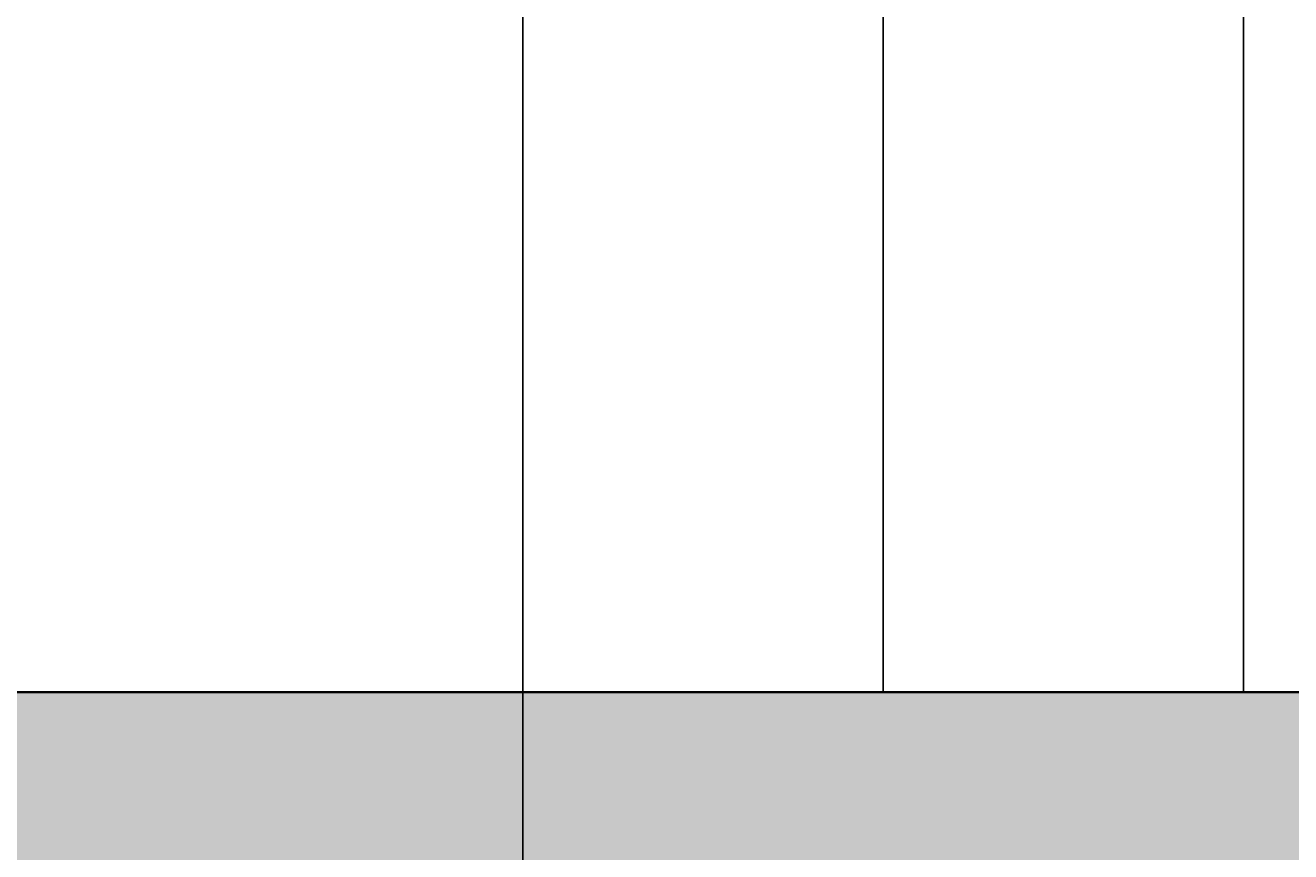
# Model space of a CAD drawing. Units: inches. Extents: x 1998 to 2588, y 1139 to 1977.
# Tile 87 of 134: x 2397 to 2425, y 1477 to 1496. Entities that reach past the tile are written whole.
import ezdxf

# ---------------------------------------------------------------- set-up
doc = ezdxf.new("R2010")
doc.units = ezdxf.units.IN
for name, color, linetype, lineweight in [('A-ANNO-DIMS', 2, 'Continuous', 18), ('A-FLOR-STRS', 7, 'Continuous', 25), ('A-WALL-PATT', 252, 'Continuous', 13), ('WALL', 200, 'Continuous', 35)]:
    doc.layers.add(name, color=color, linetype=linetype, lineweight=lineweight)
doc.styles.get("Standard").update_dxf_attribs({"font": 'arial.ttf'})
doc.dimstyles.get("Standard").update_dxf_attribs({"dimtxt": 0.18, "dimasz": 0.18, "dimexe": 0.18, "dimexo": 0.0625, "dimgap": 0.09, "dimtad": 0, "dimtih": 1, "dimtoh": 1, "dimdec": 4, "dimzin": 0, "dimdsep": 46, "dimtxsty": 'Standard', "dimcen": 0.09, "dimadec": 0, "dimazin": 0, "dimtfac": 1, "dimtdec": 4, "dimtofl": 0, "dimtmove": 0, "dimatfit": 3, "dimfxl": 1, "dimtolj": 1, "dimtzin": 0, "dimarcsym": 0})

# ---------------------------------------------------------------- blocks, each defined once
blk = doc.blocks.new('*D24')
at = {"layer": 'A-ANNO-DIMS', "color": 0, "lineweight": -2, "transparency": 16777216}
for p, q in [((2398.535, 1911.232), (2588.309, 1911.232)), ((2588.129, 1911.052), (2588.129, 1570.164)), ((2588.129, 1228.912), (2588.129, 1569.8)), ((2527.535, 1228.732), (2588.309, 1228.732))]:
    blk.add_line(p, q, dxfattribs=at)
at = {"layer": 'A-ANNO-DIMS', "color": 0, "transparency": 16777216}
for points in [[(2588.099, 1911.052), (2588.159, 1911.052), (2588.129, 1911.232)], [(2588.099, 1228.912), (2588.159, 1228.912), (2588.129, 1228.732)]]:
    blk.add_solid(points, dxfattribs=at)
at = {"layer": 'Defpoints', "color": 0, "transparency": 16777216}
for p in [(2398.473, 1911.232), (2588.129, 1911.232), (2527.473, 1228.732)]:
    blk.add_point(p, dxfattribs=at)
at = {"layer": 'A-ANNO-DIMS', "color": 0, "transparency": 16777216, "insert": (2588.129, 1569.982), "char_height": 0.18, "attachment_point": 5}
blk.add_mtext('\\A1;682.5', dxfattribs=at)
blk = doc.blocks.new('*D33')
at = {"layer": 'A-ANNO-DIMS', "color": 0, "lineweight": -2, "transparency": 16777216}
for p, q in [((2407.973, 1480.67), (2407.973, 1138.602)), ((2498.179, 1480.67), (2498.179, 1138.602)), ((2408.153, 1138.782), (2452.753, 1138.782)), ((2497.999, 1138.782), (2453.399, 1138.782))]:
    blk.add_line(p, q, dxfattribs=at)
at = {"layer": 'A-ANNO-DIMS', "color": 0, "transparency": 16777216}
for points in [[(2408.153, 1138.812), (2408.153, 1138.752), (2407.973, 1138.782)], [(2497.999, 1138.812), (2497.999, 1138.752), (2498.179, 1138.782)]]:
    blk.add_solid(points, dxfattribs=at)
at = {"layer": 'Defpoints', "color": 0, "transparency": 16777216}
for p in [(2407.973, 1480.732), (2498.179, 1480.732), (2498.179, 1138.782)]:
    blk.add_point(p, dxfattribs=at)
at = {"layer": 'A-ANNO-DIMS', "color": 0, "transparency": 16777216, "insert": (2453.076, 1138.782), "char_height": 0.18, "attachment_point": 5}
blk.add_mtext('\\A1;90.2', dxfattribs=at)
blk = doc.blocks.new('*D43')
at = {"layer": 'A-ANNO-DIMS', "color": 0, "lineweight": -2, "transparency": 16777216}
for p, q in [((2407.973, 1594.67), (2407.973, 1138.602)), ((2345.973, 1588.67), (2345.973, 1138.602)), ((2346.153, 1138.782), (2376.754, 1138.782)), ((2407.793, 1138.782), (2377.191, 1138.782))]:
    blk.add_line(p, q, dxfattribs=at)
at = {"layer": 'A-ANNO-DIMS', "color": 0, "transparency": 16777216}
for points in [[(2346.153, 1138.812), (2346.153, 1138.752), (2345.973, 1138.782)], [(2407.793, 1138.812), (2407.793, 1138.752), (2407.973, 1138.782)]]:
    blk.add_solid(points, dxfattribs=at)
at = {"layer": 'Defpoints', "color": 0, "transparency": 16777216}
for p in [(2407.973, 1594.732), (2345.973, 1588.732), (2407.973, 1138.782)]:
    blk.add_point(p, dxfattribs=at)
at = {"layer": 'A-ANNO-DIMS', "color": 0, "transparency": 16777216, "insert": (2376.973, 1138.782), "char_height": 0.18, "attachment_point": 5}
blk.add_mtext('\\A1;62', dxfattribs=at)

msp = doc.modelspace()

# ---------------------------------------------------------------- hatches: boundary and pattern name
at = {"layer": 'A-WALL-PATT'}
h = msp.add_hatch(color=256, dxfattribs=at)
h.dxf.hatch_style = 1
h.paths.add_polyline_path([(2527.4729, 1362.2324), (2510.9729, 1362.2324), (2510.9729, 1357.7324), (2518.4729, 1357.7324), (2518.4729, 1237.7324), (2503.1458, 1237.7324), (2503.1458, 1228.7324), (2527.4729, 1228.7324)])
h.paths.add_polyline_path([(2490.5682, 1362.2324), (2398.4729, 1362.2324), (2398.4729, 1357.7324), (2490.5682, 1357.7324)])
h.paths.add_polyline_path([(2224.9729, 1264.7324), (2222.9729, 1264.7324), (2222.9729, 1232.4125), (2341.4729, 1232.4125), (2341.4729, 1234.4125), (2224.9729, 1234.4125)])
h.paths.add_polyline_path([(2334.5332, 1273.7324), (2264.7638, 1273.7324), (2264.7638, 1269.5611, -0.043659), (2264.3413, 1264.7324), (2334.5332, 1264.7324)])
h.paths.add_polyline_path([(2236.9551, 1273.7324), (2234.4125, 1273.7324), (2234.4125, 1264.7324), (2236.9551, 1264.7324), (2236.9551, 1269.5611)])
h.paths.add_polyline_path([(2222.9729, 1293.2324), (2096.9729, 1293.2324), (2096.9729, 1345.0966), (2087.9729, 1345.0966), (2087.9729, 1284.2324), (2222.9729, 1284.2324), (2222.9729, 1285.137)])
h.paths.add_polyline_path([(2096.9729, 1458.7927), (2087.9729, 1458.7927), (2087.9729, 1417.7324), (2087.9729, 1413.2324), (2096.9729, 1413.2324), (2096.9729, 1417.7324)])
h.paths.add_polyline_path([(2096.9729, 1413.2324), (2087.9729, 1413.2324), (2087.9729, 1365.5012), (2096.9729, 1365.5012), (2096.9729, 1369.3358)])
h.paths.add_polyline_path([(2186.2943, 1417.7324), (2138.6074, 1417.7324), (2096.9729, 1417.7324), (2096.9729, 1413.2324), (2138.6074, 1413.2324), (2186.2943, 1413.2324)])
h.paths.add_polyline_path([(2181.4729, 1465.7324), (2176.9729, 1465.7324), (2176.9729, 1451.6434), (2181.4729, 1451.6434)])
h.paths.add_polyline_path([(2181.4729, 1422.1664), (2176.9729, 1422.1664), (2176.9729, 1417.7324), (2181.4729, 1417.7324)])
h.paths.add_polyline_path([(2063.9729, 1465.7324), (2087.9729, 1465.7324), (2087.9729, 1470.2324), (2059.4729, 1470.2324), (2059.4729, 1413.2324), (2087.9729, 1413.2324), (2087.9729, 1417.7324), (2063.9729, 1417.7324)])
h.paths.add_polyline_path([(2181.4729, 1755.2324), (2176.9729, 1755.2324), (2176.9729, 1748.6798), (2177.0513, 1748.6798), (2181.4729, 1748.6798)])
h.paths.add_polyline_path([(2227.4729, 1707.2324), (2220.4647, 1707.2324), (2220.4647, 1702.7324), (2222.9729, 1702.7324), (2222.9729, 1604.637), (2227.4729, 1604.637)])
h.paths.add_polyline_path([(2114.9729, 1702.7324), (2105.9729, 1702.7324), (2105.9729, 1628.4781, -0.0318759), (2110.1012, 1628.7416), (2114.9729, 1628.7416)])
h.paths.add_polyline_path([(2345.9729, 1739.3278), (2341.4729, 1739.3278), (2341.4729, 1647.5211), (2345.9729, 1647.5211)])
h.paths.add_polyline_path([(2350.6273, 1641.2324), (2345.9729, 1641.2324), (2345.9729, 1636.7324), (2350.6273, 1636.7324), (2350.6273, 1639.8729)])
h.paths.add_polyline_path([(2501.9729, 1641.2324), (2407.9729, 1641.2324), (2392.5005, 1641.2324), (2392.5005, 1639.8729), (2392.5005, 1636.7324), (2501.9729, 1636.7324)])
h.paths.add_polyline_path([(2510.9729, 1755.2324), (2501.9729, 1755.2324), (2501.9729, 1641.2324), (2510.9729, 1641.2324)])
h.paths.add_polyline_path([(2549.1786, 1641.2324), (2522.3775, 1641.2324), (2522.3775, 1636.7324), (2540.1786, 1636.7324), (2540.1786, 1480.7324), (2522.3775, 1480.7324), (2522.3775, 1476.2324), (2549.1786, 1476.2324)])
h.paths.add_polyline_path([(2498.1786, 1594.7324), (2407.9729, 1594.7324), (2407.9729, 1585.7324), (2416.9729, 1585.7324), (2489.1786, 1585.7324), (2489.1786, 1531.7324), (2416.9729, 1531.7324), (2407.9729, 1531.7324), (2407.9729, 1522.7324), (2498.1786, 1522.7324)])
h.paths.add_polyline_path([(2351.6437, 1480.7324), (2345.9729, 1480.7324), (2345.9729, 1476.2324), (2351.6437, 1476.2324), (2351.6437, 1477.5919)])
h.paths.add_polyline_path([(2501.9729, 1480.7324), (2498.1786, 1480.7324), (2407.9729, 1480.7324), (2393.5168, 1480.7324), (2393.5168, 1477.5919), (2393.5168, 1476.2324), (2501.9729, 1476.2324)])

# ---------------------------------------------------------------- linework, layer by layer
at = {"layer": 'A-FLOR-STRS'}
for p, q in [((2407.9729, 1480.7324), (2407.9729, 1636.7324)), ((2407.9729, 1480.7324), (2407.9729, 1522.7324)), ((2415.9729, 1480.7324), (2415.9729, 1522.7324)), ((2423.9729, 1480.7324), (2423.9729, 1522.7324))]:
    msp.add_line(p, q, dxfattribs=at)
at = {"layer": 'WALL'}
for p in [(2393.5168, 1480.7324), (2540.1786, 1480.7324)]:
    msp.add_line(p, (2407.9729, 1480.7324), dxfattribs=at)

# ---------------------------------------------------------------- dimensions: what is measured, and where the dimension line sits
at = {"layer": 'A-ANNO-DIMS'}
dim = msp.add_linear_dim(base=(2588.1286, 1911.2324), p1=(2527.4729, 1228.7324), p2=(2398.4729, 1911.2324), angle=90, dimstyle='Standard', override={"dimdec": 1, "dimlfac": 1, "dimrnd": 0, "dimzin": 0, "dimdsep": 46, "dimlunit": 2}, dxfattribs=at)
dim.commit()
dim.dimension.update_dxf_attribs({"geometry": '*D24', "text_midpoint": (2588.1286, 1569.9824)})
for base, p1, p2, override, picture, middle in [((2407.9729, 1138.7824), (2345.9729, 1588.7324), (2407.9729, 1594.7324), {"dimdec": 0, "dimlfac": 1, "dimrnd": 0, "dimzin": 0, "dimdsep": 46, "dimlunit": 2}, '*D43', (2376.9729, 1138.7824)), ((2498.1786, 1138.7824), (2407.9729, 1480.7324), (2498.1786, 1480.7324), {"dimdec": 1, "dimlfac": 1, "dimrnd": 0, "dimzin": 0, "dimdsep": 46, "dimlunit": 2}, '*D33', (2453.0757, 1138.7824))]:
    dim = msp.add_linear_dim(base=base, p1=p1, p2=p2, dimstyle='Standard', override=override, dxfattribs=at)
    dim.commit()
    dim.dimension.update_dxf_attribs({"geometry": picture, "text_midpoint": middle})

doc.saveas('drawing.dxf')
